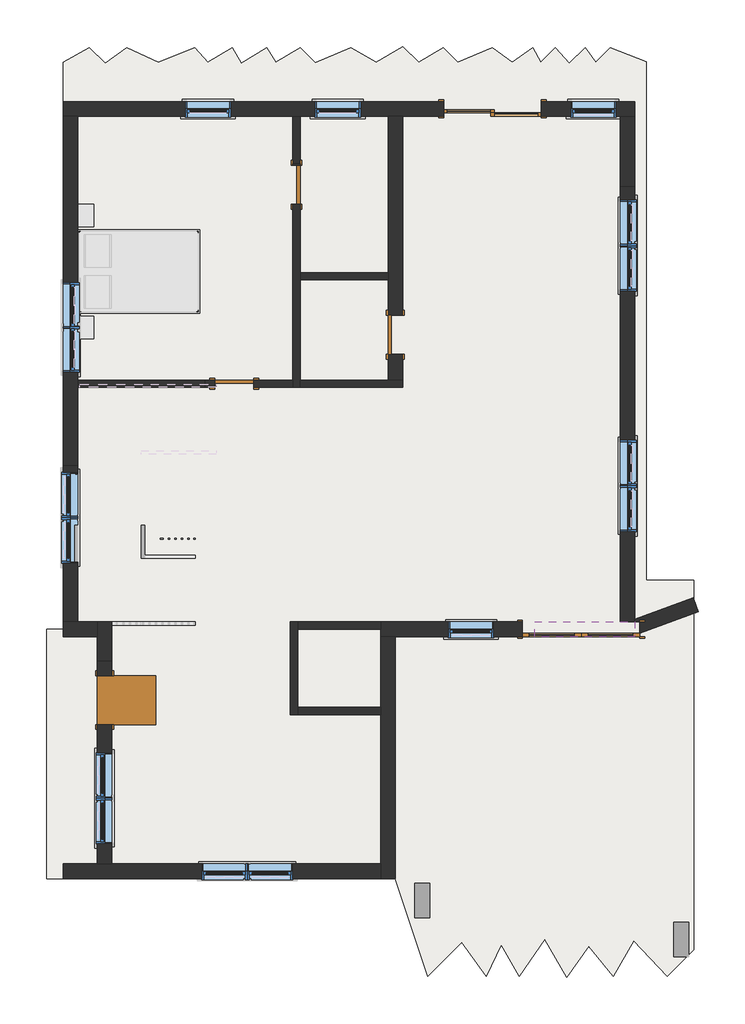
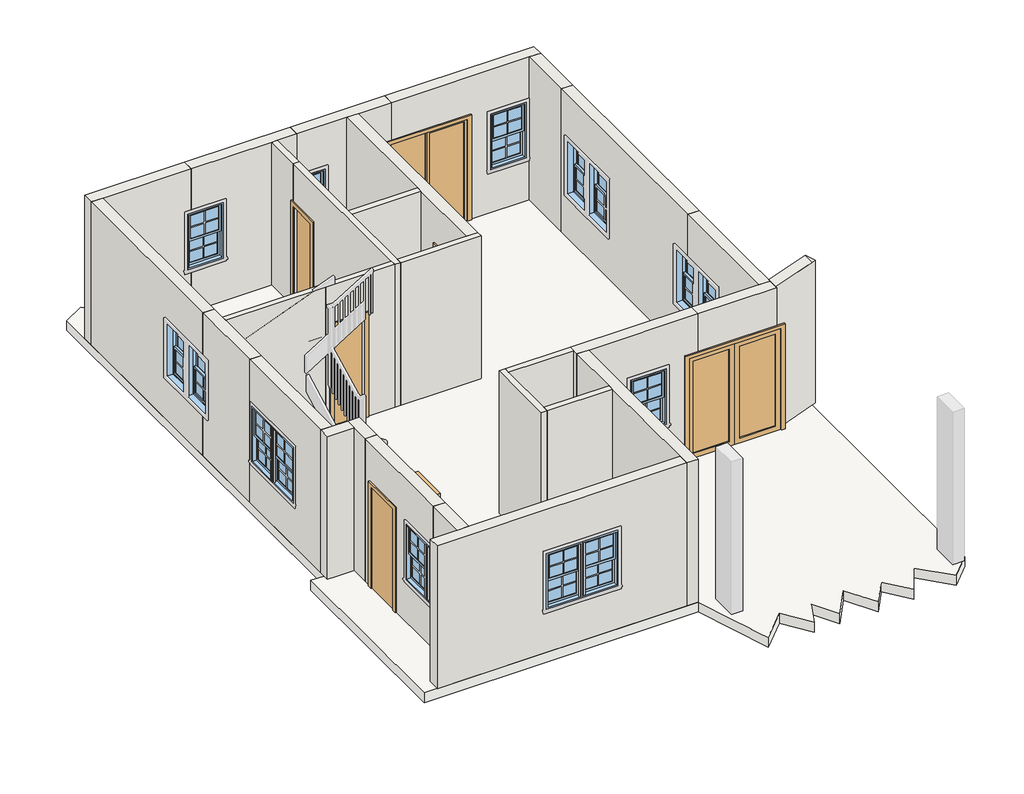
# One storey, part 1 of 3: 29 walls, 16 windows, 6 doors, 1 slab.
"""IFC4 building model written with IfcOpenShell, lengths in millimetres."""

from ifc_helpers import new_model, si_unit, frame, origin, place, context, project, spatial, polyline, outline, extrude, faceted_brep, transform, mapped, element, save
from components import door_5cbd26dd, door_238c678e, single_flush_2_x_7_f433b8c7, door_0bf9f8da, door_0d3b4037, window_fc4bf0c6

model = new_model("IFC4")

# Units and contexts
model_context = context("Model", 3, world=origin())
ifc_project = project(units=[si_unit("LENGTHUNIT", "METRE", prefix="MILLI")], contexts=[model_context])

# Site, building, storey
site = spatial("IfcSite", under=ifc_project)
building = spatial("IfcBuilding", under=site)
storey = spatial("IfcBuildingStorey", under=building, Elevation=3200.4)

# Doors
placement = place(None, origin())
door_shape = door_5cbd26dd(model_context)
element("IfcDoor", 1, ObjectType="Door-Double-Glass : 72\" x 84\"", at=placement, inside=storey, context=model_context, shape_type="MappedRepresentation", body=[
    mapped(door_shape, transform((-14398.9750992, 4551.4036146, 3200.4), x_axis=(-1.0, 0.0, 0.0), y_axis=(0.0, -1.0, 0.0), z_axis=(0.0, 0.0, 1.0))),
])
door_2_shape = door_238c678e(model_context)
element("IfcDoor", 2, ObjectType="Door-Double-Sliding : 60\" x 84\"", at=placement, inside=storey, context=model_context, shape_type="MappedRepresentation", body=[
    mapped(door_2_shape, transform((-15781.8310804, 12791.3223147, 3200.4), x_axis=(-1.0, 0.0, 0.0), y_axis=(0.0, -1.0, 0.0), z_axis=(0.0, 0.0, 1.0))),
])
single_flush_2_x_7_shape = single_flush_2_x_7_f433b8c7(model_context)
element("IfcDoor", 3, ObjectType="Single-Flush : 2' x 7'", at=placement, inside=storey, context=model_context, shape_type="MappedRepresentation", body=[
    mapped(single_flush_2_x_7_shape, transform((-21828.4750314, 3444.1223646, 3200.4), x_axis=(0.0, 1.0, 0.0), y_axis=(-1.0, 0.0, 0.0), z_axis=(0.0, 0.0, 1.0))),
])
door_3_shape = door_0bf9f8da(model_context)
element("IfcDoor", 4, ObjectType="Single-Flush : 24\" x 84\"", at=placement, inside=storey, context=model_context, shape_type="MappedRepresentation", body=[
    mapped(door_3_shape, transform((-18837.6250314, 11478.1423646, 3200.4), x_axis=(0.0, 1.0, 0.0), y_axis=(-1.0, 0.0, 0.0), z_axis=(0.0, 0.0, 1.0))),
])
element("IfcDoor", 5, ObjectType="Single-Flush : 24\" x 84\"", at=placement, inside=storey, context=model_context, shape_type="MappedRepresentation", body=[
    mapped(door_3_shape, transform((-19809.1750314, 8378.0723646, 3200.4), x_axis=(-1.0, 0.0, 0.0), y_axis=(0.0, -1.0, 0.0), z_axis=(0.0, 0.0, 1.0))),
])
door_4_shape = door_0d3b4037(model_context)
element("IfcDoor", 6, ObjectType="Single-Flush : 24\" x 84\"", at=placement, inside=storey, context=model_context, shape_type="MappedRepresentation", body=[
    mapped(door_4_shape, transform((-17294.5750314, 9140.0723646, 3200.4), x_axis=(0.0, 1.0, 0.0), y_axis=(-1.0, 0.0, 0.0), z_axis=(0.0, 0.0, 1.0))),
])

# Slab
element("IfcSlab", 7, ObjectType="LW Concrete on Metal Deck", at=placement, inside=storey, context=model_context, shape_type="SweptSolid", body=[
    extrude(outline(polyline([(-21820.2943548, 13371.8353173), (-21483.0986122, 13616.8223646), (-20992.8643301, 13388.2223646), (-20427.0594754, 13616.8223646), (-20220.0943548, 13388.2223646), (-19839.6400652, 13616.8223646), (-19695.738427, 13377.3298208), (-19297.1559002, 13616.8223646), (-19159.7991627, 13388.2223646), (-18779.344873, 13616.8223646), (-18543.6943548, 13381.1718464), (-17988.5365241, 13616.8223646), (-17592.5897095, 13388.2223646), (-17180.2750314, 13635.9660173), (-16932.5313787, 13388.2223646), (-16552.077089, 13616.8223646), (-16323.477089, 13388.2223646), (-15784.9292382, 13616.8223646), (-15470.2883312, 13388.2223646), (-15155.6474241, 13616.8223646), (-15028.932375, 13388.2223646), (-14800.332375, 13616.8223646), (-14581.2943548, 13373.5559982), (-14338.0279884, 13616.8223646), (-14171.9403665, 13388.2223646), (-13943.3403665, 13616.8223646), (-13382.9750314, 13401.7182659), (-13382.9750314, 5311.0223722), (-12646.3750314, 5311.0223722), (-12646.3750314, -450.2583119), (-13057.2943548, -861.1776354), (-13577.9943548, -311.251504), (-13895.4943548, -861.1776354), (-14276.4943548, -390.1805798), (-14619.3943548, -879.8925313), (-14962.2943548, -285.9723094), (-15365.0574601, -861.1776354), (-15648.0943548, -370.9433534), (-15876.6943548, -861.1776354), (-16257.6943548, -327.7776354), (-16791.0943548, -861.1776354), (-17294.5750314, 662.8223646), (-22734.6943548, 662.8223646), (-22734.6943548, 4549.0223646), (-22476.1752061, 4549.0223646), (-22476.1752061, 13388.2223646), (-22065.2814022, 13616.8223646), (-21820.2943548, 13371.8353173)])), frame((0.0, 0.0, 2997.2), z_axis=(0.0, 0.0, 1.0), x_axis=(1.0, 0.0, 0.0)), (0.0, 0.0, 1.0), 203.2),
])

# Walls
element("IfcWall", 8, ObjectType="Generic - 4.5\"", at=placement, inside=storey, context=model_context, shape_type="SweptSolid", body=[
    extrude(outline(polyline([(-18894.7750314, 11808.3423646), (-18894.7750314, 12550.0223147), (-18780.4750314, 12550.0223147), (-18780.4750314, 11808.3423646), (-18894.7750314, 11808.3423646)])), frame((0.0, 0.0, 3200.4), z_axis=(0.0, 0.0, 1.0), x_axis=(1.0, 0.0, 0.0)), (0.0, 0.0, 1.0), 2997.2),
])
element("IfcWall", 9, ObjectType="Generic - 4.5\"", at=placement, inside=storey, context=model_context, shape_type="Brep", body=[
    faceted_brep([(-18894.7750314, 11808.3423646, 3200.4), (-18894.7750314, 11782.9423646, 3200.4), (-18894.7750314, 11782.9423646, 5334.0), (-18894.7750314, 11173.3423646, 5334.0), (-18894.7750314, 11173.3423646, 3200.4), (-18894.7750314, 8435.2223646, 3200.4), (-18894.7750314, 8320.9223646, 3200.4), (-18894.7750314, 8320.9223646, 6197.6), (-18894.7750314, 8435.2223646, 6197.6), (-18894.7750314, 11808.3423646, 6197.6), (-18780.4750314, 11782.9423646, 5334.0), (-18780.4750314, 11782.9423646, 3200.4), (-18780.4750314, 11808.3423646, 3200.4), (-18780.4750314, 11808.3423646, 6197.6), (-18780.4750314, 10111.6223646, 6197.6), (-18780.4750314, 9997.3223646, 6197.6), (-18780.4750314, 8435.2223646, 6197.6), (-18780.4750314, 8320.9223646, 6197.6), (-18780.4750314, 8320.9223646, 3200.4), (-18780.4750314, 8435.2223646, 3200.4), (-18780.4750314, 9997.3223646, 3200.4), (-18780.4750314, 10111.6223646, 3200.4), (-18780.4750314, 11173.3423646, 3200.4), (-18780.4750314, 11173.3423646, 5334.0)], [[[0, 1, 2, 3, 4, 5, 6, 7, 8, 9]], [[10, 11, 12, 13, 14, 15, 16, 17, 18, 19, 20, 21, 22, 23]], [[12, 11, 1, 0]], [[22, 21, 20, 19, 18, 6, 5, 4]], [[0, 9, 13, 12]], [[7, 6, 18, 17]], [[2, 1, 11, 10]], [[3, 2, 10, 23]], [[4, 3, 23, 22]], [[9, 8, 7, 17, 16, 15, 14, 13]]]),
])
element("IfcWall", 10, ObjectType="Generic - 4.5\"", at=placement, inside=storey, context=model_context, shape_type="Brep", body=[
    faceted_brep([(-18780.4750314, 8320.9223646, 3200.4), (-17180.2750314, 8320.9223646, 3200.4), (-17180.2750314, 8320.9223646, 6197.6), (-18780.4750314, 8320.9223646, 6197.6), (-18780.4750314, 8435.2223646, 3200.4), (-18780.4750314, 8435.2223646, 6197.6), (-17408.8750314, 8435.2223646, 6197.6), (-17180.2750314, 8435.2223646, 6197.6), (-17180.2750314, 8435.2223646, 3200.4), (-17408.8750314, 8435.2223646, 3200.4)], [[[0, 1, 2, 3]], [[4, 5, 6, 7, 8, 9]], [[1, 0, 4, 9, 8]], [[0, 3, 5, 4]], [[2, 1, 8, 7]], [[3, 2, 7, 6, 5]]]),
])
element("IfcWall", 11, ObjectType="Generic - 4.5\"", at=placement, inside=storey, context=model_context, shape_type="SweptSolid", body=[
    extrude(outline(polyline([(3200.4, -20266.3750314), (3200.4, -20113.9750314), (5334.0, -20113.9750314), (5334.0, -19504.3750314), (3200.4, -19504.3750314), (3200.4, -18894.7750314), (6197.6, -18894.7750314), (6197.6, -20266.3750314), (3200.4, -20266.3750314)])), frame((0.0, 8320.9223646, 0.0), z_axis=(0.0, 1.0, 0.0), x_axis=(0.0, 0.0, 1.0)), (0.0, 0.0, 1.0), 114.3),
])
element("IfcWall", 12, ObjectType="Generic - 4.5\"", at=placement, inside=storey, context=model_context, shape_type="SweptSolid", body=[
    extrude(outline(polyline([(-20266.3750314, 8320.9223646), (-22247.5752061, 8320.9223646), (-22247.5752061, 8435.2223646), (-20266.3750314, 8435.2223646), (-20266.3750314, 8320.9223646)])), frame((0.0, 0.0, 3200.4), z_axis=(0.0, 0.0, 1.0), x_axis=(1.0, 0.0, 0.0)), (0.0, 0.0, 1.0), 2997.2),
])
element("IfcWall", 13, ObjectType="Generic - 4.5\"", at=placement, inside=storey, context=model_context, shape_type="SweptSolid", body=[
    extrude(outline(polyline([(-17408.8750314, 9997.3223646), (-18780.4750314, 9997.3223646), (-18780.4750314, 10111.6223646), (-17408.8750314, 10111.6223646), (-17408.8750314, 9997.3223646)])), frame((0.0, 0.0, 3200.4), z_axis=(0.0, 0.0, 1.0), x_axis=(1.0, 0.0, 0.0)), (0.0, 0.0, 1.0), 2997.2),
])
element("IfcWall", 14, ObjectType="Generic - 4.5\"", at=placement, inside=storey, context=model_context, shape_type="Brep", body=[
    faceted_brep([(-18932.8750314, 4663.3223646, 3200.4), (-18932.8750314, 3215.5223646, 3200.4), (-18932.8750314, 3215.5223646, 6197.6), (-18932.8750314, 4663.3223646, 6197.6), (-18818.5750314, 4663.3223646, 3200.4), (-18818.5750314, 4663.3223646, 6197.6), (-18818.5750314, 4549.0223646, 6197.6), (-18818.5750314, 3329.8223646, 6197.6), (-18818.5750314, 3215.5223646, 6197.6), (-18818.5750314, 3215.5223646, 3200.4), (-18818.5750314, 3329.8223646, 3200.4), (-18818.5750314, 4549.0223646, 3200.4)], [[[0, 1, 2, 3]], [[4, 5, 6, 7, 8, 9, 10, 11]], [[1, 0, 4, 11, 10, 9]], [[2, 1, 9, 8]], [[0, 3, 5, 4]], [[3, 2, 8, 7, 6, 5]]]),
])
element("IfcWall", 15, ObjectType="Generic - 4.5\"", at=placement, inside=storey, context=model_context, shape_type="SweptSolid", body=[
    extrude(outline(polyline([(-17523.1750314, 3215.5223646), (-18818.5750314, 3215.5223646), (-18818.5750314, 3329.8223646), (-17523.1750314, 3329.8223646), (-17523.1750314, 3215.5223646)])), frame((0.0, 0.0, 3200.4), z_axis=(0.0, 0.0, 1.0), x_axis=(1.0, 0.0, 0.0)), (0.0, 0.0, 1.0), 2997.2),
])
element("IfcWall", 16, ObjectType="Generic - 4.5\"", at=placement, inside=storey, context=model_context, shape_type="SweptSolid", body=[
    extrude(outline(polyline([(-17523.1750314, 4549.0223646), (-18818.5750314, 4549.0223646), (-18818.5750314, 4663.3223646), (-17523.1750314, 4663.3223646), (-17523.1750314, 4549.0223646)])), frame((0.0, 0.0, 3200.4), z_axis=(0.0, 0.0, 1.0), x_axis=(1.0, 0.0, 0.0)), (0.0, 0.0, 1.0), 2997.2),
])
element("IfcWall", 17, ObjectType="Generic -9\"Brick 2", at=placement, inside=storey, context=model_context, shape_type="Brep", body=[
    faceted_brep([(-22476.1750314, 12550.0223646, 3200.4), (-22247.5750314, 12550.0223646, 3200.4), (-20494.9750314, 12550.0223646, 3200.4), (-20494.9750314, 12550.0223646, 4114.8), (-20571.1750314, 12550.0223646, 4114.8), (-20571.1750314, 12550.0223646, 5283.2), (-20494.9750314, 12550.0223646, 5283.2), (-20494.9750314, 12550.0223646, 6197.6), (-22247.5750314, 12550.0223646, 6197.6), (-22476.1752061, 12550.0223646, 6197.6), (-20494.9750314, 12778.6223646, 3200.4), (-22476.1750314, 12778.6223646, 3200.4), (-22476.1750314, 12778.6223646, 6197.6), (-20494.9750314, 12778.6223646, 6197.6), (-20494.9750314, 12778.6223646, 5283.2), (-20571.1750314, 12778.6223646, 5283.2), (-20571.1750314, 12778.6223646, 4114.8), (-20494.9750314, 12778.6223646, 4114.8)], [[[0, 1, 2, 3, 4, 5, 6, 7, 8, 9]], [[10, 11, 12, 13, 14, 15, 16, 17]], [[2, 1, 0, 11, 10]], [[2, 10, 17, 3]], [[13, 7, 6, 14]], [[0, 9, 12, 11]], [[16, 4, 3, 17]], [[4, 16, 15, 5]], [[5, 15, 14, 6]], [[9, 8, 7, 13, 12]]]),
])
element("IfcWall", 18, ObjectType="Generic -9\"Brick 2", at=placement, inside=storey, context=model_context, shape_type="Brep", body=[
    faceted_brep([(-20494.9750314, 12550.0223147, 3200.4), (-18894.7750314, 12550.0223147, 3200.4), (-18780.4750314, 12550.0223147, 3200.4), (-18397.0494379, 12550.0223147, 3200.4), (-18397.0494379, 12550.0223147, 4114.8), (-18549.4494379, 12550.0223147, 4114.8), (-18549.4494379, 12550.0223147, 5283.2), (-18397.0494379, 12550.0223147, 5283.2), (-18397.0494379, 12550.0223147, 6197.6), (-18780.4750314, 12550.0223147, 6197.6), (-18894.7750314, 12550.0223147, 6197.6), (-20494.9750314, 12550.0223147, 6197.6), (-20494.9750314, 12550.0223147, 5283.2), (-19859.9750314, 12550.0223147, 5283.2), (-19859.9750314, 12550.0223147, 4114.8), (-20494.9750314, 12550.0223147, 4114.8), (-18397.0494379, 12778.6223147, 3200.4), (-20494.9750314, 12778.6223147, 3200.4), (-20494.9750314, 12778.6223147, 4114.8), (-19859.9750314, 12778.6223147, 4114.8), (-19859.9750314, 12778.6223147, 5283.2), (-20494.9750314, 12778.6223147, 5283.2), (-20494.9750314, 12778.6223147, 6197.6), (-18397.0494379, 12778.6223147, 6197.6), (-18397.0494379, 12778.6223147, 5283.2), (-18549.4494379, 12778.6223147, 5283.2), (-18549.4494379, 12778.6223147, 4114.8), (-18397.0494379, 12778.6223147, 4114.8)], [[[0, 1, 2, 3, 4, 5, 6, 7, 8, 9, 10, 11, 12, 13, 14, 15]], [[16, 17, 18, 19, 20, 21, 22, 23, 24, 25, 26, 27]], [[3, 2, 1, 0, 17, 16]], [[3, 16, 27, 4]], [[23, 8, 7, 24]], [[17, 0, 15, 18]], [[12, 11, 22, 21]], [[13, 20, 19, 14]], [[14, 19, 18, 15]], [[20, 13, 12, 21]], [[26, 5, 4, 27]], [[5, 26, 25, 6]], [[6, 25, 24, 7]], [[11, 10, 9, 8, 23, 22]]]),
])
element("IfcWall", 19, ObjectType="Generic -9\"Brick 2", at=placement, inside=storey, context=model_context, shape_type="Brep", body=[
    faceted_brep([(-18397.0494379, 12550.0223147, 4114.8), (-18397.0494379, 12550.0223147, 3200.4), (-17408.8750314, 12550.0223147, 3200.4), (-17180.2750314, 12550.0223147, 3200.4), (-16543.8310804, 12550.0223147, 3200.4), (-16543.8310804, 12550.0223147, 5334.0), (-16518.4310804, 12550.0223147, 5334.0), (-16518.4310804, 12550.0223147, 6197.6), (-17180.2750314, 12550.0223147, 6197.6), (-17408.8750314, 12550.0223147, 6197.6), (-18397.0494379, 12550.0223147, 6197.6), (-18397.0494379, 12550.0223147, 5283.2), (-17838.2494379, 12550.0223147, 5283.2), (-17838.2494379, 12550.0223147, 4114.8), (-18397.0494379, 12778.6223147, 3200.4), (-18397.0494379, 12778.6223147, 4114.8), (-17838.2494379, 12778.6223147, 4114.8), (-17838.2494379, 12778.6223147, 5283.2), (-18397.0494379, 12778.6223147, 5283.2), (-18397.0494379, 12778.6223147, 6197.6), (-16518.4310804, 12778.6223147, 6197.6), (-16518.4310804, 12778.6223147, 5334.0), (-16543.8310804, 12778.6223147, 5334.0), (-16543.8310804, 12778.6223147, 3200.4)], [[[0, 1, 2, 3, 4, 5, 6, 7, 8, 9, 10, 11, 12, 13]], [[14, 15, 16, 17, 18, 19, 20, 21, 22, 23]], [[1, 14, 23, 4, 3, 2]], [[20, 7, 6, 21]], [[14, 1, 0, 15]], [[11, 10, 19, 18]], [[12, 17, 16, 13]], [[13, 16, 15, 0]], [[17, 12, 11, 18]], [[22, 5, 4, 23]], [[5, 22, 21, 6]], [[10, 9, 8, 7, 20, 19]]]),
])
element("IfcWall", 20, ObjectType="Generic -9\"Brick 2", at=placement, inside=storey, context=model_context, shape_type="Brep", body=[
    faceted_brep([(-13560.7750314, 12550.0223147, 3200.4), (-13560.7750314, 12550.0223147, 6197.6), (-13789.3750314, 12550.0223147, 6197.6), (-16518.4310804, 12550.0223147, 6197.6), (-16518.4310804, 12550.0223147, 5334.0), (-15019.8310804, 12550.0223147, 5334.0), (-15019.8310804, 12550.0223147, 3200.4), (-13789.3750314, 12550.0223147, 3200.4), (-13852.8750314, 12550.0223147, 5283.2), (-13852.8750314, 12550.0223147, 4114.8), (-14564.0750314, 12550.0223147, 4114.8), (-14564.0750314, 12550.0223147, 5283.2), (-13560.7750314, 12778.6223147, 6197.6), (-13560.7750314, 12778.6223147, 3200.4), (-15019.8310804, 12778.6223147, 3200.4), (-15019.8310804, 12778.6223147, 5334.0), (-16518.4310804, 12778.6223147, 5334.0), (-16518.4310804, 12778.6223147, 6197.6), (-13852.8750314, 12778.6223147, 5283.2), (-14564.0750314, 12778.6223147, 5283.2), (-14564.0750314, 12778.6223147, 4114.8), (-13852.8750314, 12778.6223147, 4114.8)], [[[0, 1, 2, 3, 4, 5, 6, 7], [8, 9, 10, 11]], [[12, 13, 14, 15, 16, 17], [18, 19, 20, 21]], [[13, 0, 7, 6, 14]], [[3, 17, 16, 4]], [[1, 0, 13, 12]], [[9, 8, 18, 21]], [[10, 9, 21, 20]], [[11, 10, 20, 19]], [[8, 11, 19, 18]], [[5, 15, 14, 6]], [[15, 5, 4, 16]], [[3, 2, 1, 12, 17]]]),
])
element("IfcWall", 21, ObjectType="Generic -9\"Brick 2", at=placement, inside=storey, context=model_context, shape_type="SweptSolid", body=[
    extrude(outline(polyline([(-13789.3750314, 11447.1098201), (-13789.3750314, 12550.0223147), (-13560.7750314, 12550.0223147), (-13560.7750314, 11447.1098201), (-13789.3750314, 11447.1098201)])), frame((0.0, 0.0, 3200.4), z_axis=(0.0, 0.0, 1.0), x_axis=(1.0, 0.0, 0.0)), (0.0, 0.0, 1.0), 2997.2),
])
element("IfcWall", 22, ObjectType="Generic -9\"Brick 2", at=placement, inside=storey, context=model_context, shape_type="SweptSolid", body=[
    extrude(outline(polyline([(11447.1098201, 3200.4), (7101.7223647, 3200.4), (7101.7223647, 4114.8), (7495.4223646, 4114.8), (7495.4223646, 5283.2), (7101.7223647, 5283.2), (7101.7223647, 6197.6), (11447.1098201, 6197.6), (11447.1098201, 3200.4)]), holes=[polyline([(11243.9098201, 4114.8), (11243.9098201, 5283.2), (9821.5098201, 5283.2), (9821.5098201, 4114.8), (11243.9098201, 4114.8)])]), frame((-13789.3750314, 0.0, 0.0), z_axis=(1.0, 0.0, 0.0), x_axis=(0.0, 1.0, 0.0)), (0.0, 0.0, 1.0), 228.6),
])
element("IfcWall", 23, ObjectType="Generic -9\"Brick 2", at=placement, inside=storey, context=model_context, shape_type="Brep", body=[
    faceted_brep([(-13789.3750314, 7101.7223647, 3200.4), (-13789.3750314, 4663.3223646, 3200.4), (-13789.3750314, 4663.3223646, 6197.6), (-13789.3750314, 7101.7223647, 6197.6), (-13789.3750314, 7101.7223647, 5283.2), (-13789.3750314, 6073.0223646, 5283.2), (-13789.3750314, 6073.0223646, 4114.8), (-13789.3750314, 7101.7223647, 4114.8), (-13560.7750314, 4663.3223646, 3200.4), (-13560.7750314, 4704.9241624, 3200.4), (-13560.7750314, 7101.7223647, 3200.4), (-13560.7750314, 7101.7223647, 4114.8), (-13560.7750314, 6073.0223646, 4114.8), (-13560.7750314, 6073.0223646, 5283.2), (-13560.7750314, 7101.7223647, 5283.2), (-13560.7750314, 7101.7223647, 6197.6), (-13560.7750314, 5336.4223722, 6197.6), (-13560.7750314, 4704.9241624, 6197.6), (-13560.7750314, 4663.3223646, 6197.6), (-13560.7750314, 4663.3223646, 5334.0)], [[[0, 1, 2, 3, 4, 5, 6, 7]], [[8, 9, 10, 11, 12, 13, 14, 15, 16, 17, 18, 19]], [[1, 0, 10, 9, 8]], [[10, 0, 7, 11]], [[3, 15, 14, 4]], [[2, 1, 8, 19, 18]], [[6, 12, 11, 7]], [[4, 14, 13, 5]], [[12, 6, 5, 13]], [[15, 3, 2, 18, 17, 16]]]),
])
element("IfcWall", 24, ObjectType="Generic -9\"Brick 2", at=placement, inside=storey, context=model_context, shape_type="Brep", body=[
    faceted_brep([(-13560.7750314, 4434.7223646, 6197.6), (-15122.8751671, 4434.7223646, 6197.6), (-15122.8751671, 4434.7223646, 5334.0), (-13560.7750314, 4434.7223646, 5334.0), (-15122.8751671, 4663.3223646, 6197.6), (-13789.3750314, 4663.3223646, 6197.6), (-13560.7750314, 4663.3223646, 6197.6), (-13560.7750314, 4663.3223646, 5334.0), (-15122.8751671, 4663.3223646, 5334.0), (-13560.7750314, 4461.6531236, 6197.6), (-13560.7750314, 4461.6531236, 5334.0)], [[[0, 1, 2, 3]], [[4, 5, 6, 7, 8]], [[1, 4, 8, 2]], [[6, 9, 0, 3, 10, 7]], [[3, 2, 8, 7, 10]], [[1, 0, 9, 6, 5, 4]]]),
])
element("IfcWall", 25, ObjectType="Generic -9\"Brick 2", at=placement, inside=storey, context=model_context, shape_type="Brep", body=[
    faceted_brep([(-17523.1750314, 4663.3223722, 3200.4), (-17523.1750314, 4663.3223722, 6197.6), (-15122.8751671, 4663.3223722, 6197.6), (-15122.8751671, 4663.3223722, 5334.0), (-15313.3750992, 4663.3223722, 5334.0), (-15313.3750992, 4663.3223722, 3200.4), (-15757.8750314, 4663.3223722, 5283.2), (-16469.0750314, 4663.3223722, 5283.2), (-16469.0750314, 4663.3223722, 4114.8), (-15757.8750314, 4663.3223722, 4114.8), (-17523.1750314, 4434.7223722, 6197.6), (-17523.1750314, 4434.7223722, 3200.4), (-17294.5750314, 4434.7223722, 3200.4), (-15313.3750992, 4434.7223722, 3200.4), (-15313.3750992, 4434.7223722, 5334.0), (-15122.8751671, 4434.7223722, 5334.0), (-15122.8751671, 4434.7223722, 6197.6), (-17294.5750314, 4434.7223722, 6197.6), (-15757.8750314, 4434.7223722, 5283.2), (-15757.8750314, 4434.7223722, 4114.8), (-16469.0750314, 4434.7223722, 4114.8), (-16469.0750314, 4434.7223722, 5283.2), (-17523.1750314, 4549.0223646, 3200.4), (-17523.1750314, 4549.0223646, 6197.6)], [[[0, 1, 2, 3, 4, 5], [6, 7, 8, 9]], [[10, 11, 12, 13, 14, 15, 16, 17], [18, 19, 20, 21]], [[11, 22, 0, 5, 13, 12]], [[2, 16, 15, 3]], [[1, 0, 22, 11, 10, 23]], [[4, 14, 13, 5]], [[14, 4, 3, 15]], [[19, 18, 6, 9]], [[20, 19, 9, 8]], [[21, 20, 8, 7]], [[18, 21, 7, 6]], [[2, 1, 23, 10, 17, 16]]]),
])
element("IfcWall", 26, ObjectType="Generic -9\"Brick 2", at=placement, inside=storey, context=model_context, shape_type="Brep", body=[
    faceted_brep([(-17523.1750314, 4434.7223722, 3200.4), (-17523.1750314, 3329.8223646, 3200.4), (-17523.1750314, 3215.5223646, 3200.4), (-17523.1750314, 891.4223646, 3200.4), (-17523.1750314, 662.8223646, 3200.4), (-17523.1750314, 662.8223646, 6197.6), (-17523.1750314, 891.4223646, 6197.6), (-17523.1750314, 3215.5223646, 6197.6), (-17523.1750314, 3329.8223646, 6197.6), (-17523.1750314, 4434.7223722, 6197.6), (-17294.5750314, 4434.7223722, 3200.4), (-17294.5750314, 4434.7223722, 6197.6), (-17294.5750314, 662.8223646, 6197.6), (-17294.5750314, 662.8223646, 3200.4)], [[[0, 1, 2, 3, 4, 5, 6, 7, 8, 9]], [[10, 11, 12, 13]], [[4, 3, 2, 1, 0, 10, 13]], [[0, 9, 11, 10]], [[5, 4, 13, 12]], [[9, 8, 7, 6, 5, 12, 11]]]),
])
element("IfcWall", 27, ObjectType="Generic -9\"Brick 2", at=placement, inside=storey, context=model_context, shape_type="Brep", body=[
    faceted_brep([(-17523.1750314, 891.4223646, 3200.4), (-21714.1750314, 891.4223646, 3200.4), (-21942.7750314, 891.4223646, 3200.4), (-22476.1750314, 891.4223646, 3200.4), (-22476.1750314, 891.4223646, 6197.6), (-21942.7750314, 891.4223646, 6197.6), (-21714.1750314, 891.4223646, 6197.6), (-17523.1750314, 891.4223646, 6197.6), (-18894.6931686, 891.4223646, 5283.2), (-20317.0931686, 891.4223646, 5283.2), (-20317.0931686, 891.4223646, 4114.8), (-18894.6931686, 891.4223646, 4114.8), (-22476.1750314, 662.8223646, 3200.4), (-17523.1750314, 662.8223646, 3200.4), (-17523.1750314, 662.8223646, 6197.6), (-22476.1750314, 662.8223646, 6197.6), (-20317.0931686, 662.8223646, 5283.2), (-18894.6931686, 662.8223646, 5283.2), (-18894.6931686, 662.8223646, 4114.8), (-20317.0931686, 662.8223646, 4114.8)], [[[0, 1, 2, 3, 4, 5, 6, 7], [8, 9, 10, 11]], [[12, 13, 14, 15], [16, 17, 18, 19]], [[3, 2, 1, 0, 13, 12]], [[4, 3, 12, 15]], [[0, 7, 14, 13]], [[16, 9, 8, 17]], [[18, 11, 10, 19]], [[18, 17, 8, 11]], [[19, 10, 9, 16]], [[7, 6, 5, 4, 15, 14]]]),
])
element("IfcWall", 28, ObjectType="Generic -9\"Brick 2", at=placement, inside=storey, context=model_context, shape_type="SweptSolid", body=[
    extrude(outline(polyline([(1710.5723646, 3200.4), (891.4223646, 3200.4), (891.4223646, 6197.6), (1710.5723646, 6197.6), (1710.5723646, 5283.2), (1202.5723646, 5283.2), (1202.5723646, 4114.8), (1710.5723646, 4114.8), (1710.5723646, 3200.4)])), frame((-21942.7750314, 0.0, 0.0), z_axis=(1.0, 0.0, 0.0), x_axis=(0.0, 1.0, 0.0)), (0.0, 0.0, 1.0), 228.6),
])
element("IfcWall", 29, ObjectType="Generic -9\"Brick 2", at=placement, inside=storey, context=model_context, shape_type="SweptSolid", body=[
    extrude(outline(polyline([(4053.7223646, 3200.4), (3825.1223646, 3200.4), (3825.1223646, 5334.0), (3063.1223646, 5334.0), (3063.1223646, 3200.4), (1710.5723646, 3200.4), (1710.5723646, 4114.8), (2624.9723646, 4114.8), (2624.9723646, 5283.2), (1710.5723646, 5283.2), (1710.5723646, 6197.6), (4053.7223646, 6197.6), (4053.7223646, 3200.4)])), frame((-21942.7750314, 0.0, 0.0), z_axis=(1.0, 0.0, 0.0), x_axis=(0.0, 1.0, 0.0)), (0.0, 0.0, 1.0), 228.6),
])
element("IfcWall", 30, ObjectType="Generic -9\"Brick 2", at=placement, inside=storey, context=model_context, shape_type="Brep", body=[
    faceted_brep([(-21714.1750314, 4053.7223646, 3200.4), (-21714.1750314, 4663.3223646, 3200.4), (-21714.1750314, 4663.3223646, 6197.6), (-21714.1750314, 4053.7223646, 6197.6), (-21942.7750314, 4053.7223646, 3200.4), (-21942.7750314, 4053.7223646, 6197.6), (-21942.7750314, 4434.7223646, 6197.6), (-21942.7750314, 4663.3223646, 6197.6), (-21942.7750314, 4663.3223646, 3200.4), (-21942.7750314, 4434.7223646, 3200.4)], [[[0, 1, 2, 3]], [[4, 5, 6, 7, 8, 9]], [[1, 0, 4, 9, 8]], [[0, 3, 5, 4]], [[2, 1, 8, 7]], [[3, 2, 7, 6, 5]]]),
])
element("IfcWall", 31, ObjectType="Generic -9\"Brick 2", at=placement, inside=storey, context=model_context, shape_type="SweptSolid", body=[
    extrude(outline(polyline([(12550.0223646, 3200.4), (8710.539033, 3200.4), (8710.539033, 4114.8), (9955.139033, 4114.8), (9955.139033, 5283.2), (8710.539033, 5283.2), (8710.539033, 6197.6), (12550.0223646, 6197.6), (12550.0223646, 3200.4)])), frame((-22476.1750314, 0.0, 0.0), z_axis=(1.0, 0.0, 0.0), x_axis=(0.0, 1.0, 0.0)), (0.0, 0.0, 1.0), 228.6),
])
element("IfcWall", 32, ObjectType="Generic -9\"Brick 2", at=placement, inside=storey, context=model_context, shape_type="Brep", body=[
    faceted_brep([(-22476.1752061, 8710.539033, 3200.4), (-22476.1752061, 7101.7223643, 3200.4), (-22476.1752061, 7101.7223643, 6197.6), (-22476.1752061, 8710.539033, 6197.6), (-22476.1752061, 8710.539033, 5283.2), (-22476.1752061, 8558.139033, 5283.2), (-22476.1752061, 8558.139033, 4114.8), (-22476.1752061, 8710.539033, 4114.8), (-22247.5752061, 7101.7223643, 3200.4), (-22247.5752061, 8320.9223646, 3200.4), (-22247.5752061, 8435.2223646, 3200.4), (-22247.5752061, 8710.539033, 3200.4), (-22247.5752061, 8710.539033, 4114.8), (-22247.5752061, 8558.139033, 4114.8), (-22247.5752061, 8558.139033, 5283.2), (-22247.5752061, 8710.539033, 5283.2), (-22247.5752061, 8710.539033, 6197.6), (-22247.5752061, 8435.2223646, 6197.6), (-22247.5752061, 8320.9223646, 6197.6), (-22247.5752061, 7101.7223643, 6197.6)], [[[0, 1, 2, 3, 4, 5, 6, 7]], [[8, 9, 10, 11, 12, 13, 14, 15, 16, 17, 18, 19]], [[1, 0, 11, 10, 9, 8]], [[2, 1, 8, 19]], [[11, 0, 7, 12]], [[3, 16, 15, 4]], [[6, 13, 12, 7]], [[13, 6, 5, 14]], [[14, 5, 4, 15]], [[3, 2, 19, 18, 17, 16]]]),
])
element("IfcWall", 33, ObjectType="Generic -9\"Brick 2", at=placement, inside=storey, context=model_context, shape_type="SweptSolid", body=[
    extrude(outline(polyline([(7101.7223643, 3200.4), (4663.3223646, 3200.4), (4663.3223646, 6197.6), (7101.7223643, 6197.6), (7101.7223643, 3200.4)]), holes=[polyline([(5577.7223643, 4114.8), (7000.1223643, 4114.8), (7000.1223643, 5283.2), (5577.7223643, 5283.2), (5577.7223643, 4114.8)])]), frame((-22476.1752061, 0.0, 0.0), z_axis=(1.0, 0.0, 0.0), x_axis=(0.0, 1.0, 0.0)), (0.0, 0.0, 1.0), 228.6),
])
element("IfcWall", 34, ObjectType="Generic -9\"Brick 2", at=placement, inside=storey, context=model_context, shape_type="Brep", body=[
    faceted_brep([(-22476.1752061, 4434.7223646, 3200.4), (-21942.7750314, 4434.7223646, 3200.4), (-21942.7750314, 4434.7223646, 6197.6), (-22476.1752061, 4434.7223646, 6197.6), (-22476.1752061, 4663.3223646, 3200.4), (-22476.1752061, 4663.3223646, 6197.6), (-22247.5752061, 4663.3223646, 6197.6), (-21942.7750314, 4663.3223646, 6197.6), (-21942.7750314, 4663.3223646, 3200.4), (-22247.5752061, 4663.3223646, 3200.4)], [[[0, 1, 2, 3]], [[4, 5, 6, 7, 8, 9]], [[1, 0, 4, 9, 8]], [[0, 3, 5, 4]], [[2, 1, 8, 7]], [[3, 2, 7, 6, 5]]]),
])
element("IfcWall", 35, ObjectType="Generic -9\"Brick 2", at=placement, inside=storey, context=model_context, shape_type="Brep", body=[
    faceted_brep([(-17408.8750314, 12550.0223147, 3200.4), (-17408.8750314, 10111.6223646, 3200.4), (-17408.8750314, 9997.3223646, 3200.4), (-17408.8750314, 9444.8723646, 3200.4), (-17408.8750314, 9444.8723646, 5334.0), (-17408.8750314, 8835.2723646, 5334.0), (-17408.8750314, 8835.2723646, 3200.4), (-17408.8750314, 8435.2223646, 3200.4), (-17408.8750314, 8435.2223646, 6197.6), (-17408.8750314, 9997.3223646, 6197.6), (-17408.8750314, 10111.6223646, 6197.6), (-17408.8750314, 12550.0223147, 6197.6), (-17180.2750314, 9444.8723646, 5334.0), (-17180.2750314, 9444.8723646, 3200.4), (-17180.2750314, 12550.0223147, 3200.4), (-17180.2750314, 12550.0223147, 6197.6), (-17180.2750314, 8435.2223646, 6197.6), (-17180.2750314, 8435.2223646, 3200.4), (-17180.2750314, 8835.2723646, 3200.4), (-17180.2750314, 8835.2723646, 5334.0)], [[[0, 1, 2, 3, 4, 5, 6, 7, 8, 9, 10, 11]], [[12, 13, 14, 15, 16, 17, 18, 19]], [[18, 17, 7, 6]], [[14, 13, 3, 2, 1, 0]], [[0, 11, 15, 14]], [[8, 7, 17, 16]], [[4, 3, 13, 12]], [[5, 4, 12, 19]], [[6, 5, 19, 18]], [[11, 10, 9, 8, 16, 15]]]),
])
element("IfcWall", 36, ObjectType="Generic -9\"Brick 2", at=placement, inside=storey, context=model_context, shape_type="Brep", body=[
    faceted_brep([(-12570.5569462, 4822.063032, 3200.4), (-12570.5569462, 4822.063032, 6197.6), (-12646.3750314, 4794.4675058, 6197.6), (-13560.7750314, 4461.6531236, 6197.6), (-13560.7750314, 4461.6531236, 5334.0), (-13484.5750992, 4489.3876307, 5334.0), (-13484.5750992, 4489.3876307, 3200.4), (-12648.7427509, 5036.8767651, 3200.4), (-13560.7750314, 4704.9241624, 3200.4), (-13560.7750314, 4704.9241624, 6197.6), (-12648.7427509, 5036.8767651, 6197.6), (-13484.5750992, 4663.3223646, 3200.4), (-13560.7750314, 4663.3223646, 3200.4), (-12646.3750314, 5030.3715091, 6197.6), (-13560.7750314, 4663.3223646, 5334.0), (-13560.7750314, 4663.3223646, 6197.6), (-13484.5750992, 4663.3223646, 5334.0)], [[[0, 1, 2, 3, 4, 5, 6]], [[7, 8, 9, 10]], [[8, 7, 0, 6, 11, 12]], [[1, 0, 7, 10, 13]], [[9, 8, 12, 14, 4, 3, 15]], [[16, 5, 4, 14]], [[16, 11, 6, 5]], [[11, 16, 14, 12]], [[2, 1, 13]], [[3, 2, 13, 10, 9, 15]]]),
])

# Windows
window_shape = window_fc4bf0c6(model_context)
element("IfcWindow", 37, ObjectType="Window-Double-Hung : 28\" x 46\"", at=placement, inside=storey, context=model_context, shape_type="MappedRepresentation", body=[
    mapped(window_shape, transform((-20215.5750314, 12664.3223147, 3200.4), x_axis=(-1.0, 0.0, 0.0), y_axis=(0.0, -1.0, 0.0), z_axis=(0.0, 0.0, 1.0))),
])
element("IfcWindow", 38, ObjectType="Window-Double-Hung : 28\" x 46\"", at=placement, inside=storey, context=model_context, shape_type="MappedRepresentation", body=[
    mapped(window_shape, transform((-14208.4750314, 12664.3223147, 3200.4), x_axis=(-1.0, 0.0, 0.0), y_axis=(0.0, -1.0, 0.0), z_axis=(0.0, 0.0, 1.0))),
])
element("IfcWindow", 39, ObjectType="Window-Double-Hung : 28\" x 46\"", at=placement, inside=storey, context=model_context, shape_type="MappedRepresentation", body=[
    mapped(window_shape, transform((-13675.0750314, 10888.3098201, 3200.4), x_axis=(0.0, -1.0, 0.0), y_axis=(1.0, 0.0, 0.0), z_axis=(0.0, 0.0, 1.0))),
])
element("IfcWindow", 40, ObjectType="Window-Double-Hung : 28\" x 46\"", at=placement, inside=storey, context=model_context, shape_type="MappedRepresentation", body=[
    mapped(window_shape, transform((-13675.0750314, 10177.1098201, 3200.4), x_axis=(0.0, -1.0, 0.0), y_axis=(1.0, 0.0, 0.0), z_axis=(0.0, 0.0, 1.0))),
])
element("IfcWindow", 41, ObjectType="Window-Double-Hung : 28\" x 46\"", at=placement, inside=storey, context=model_context, shape_type="MappedRepresentation", body=[
    mapped(window_shape, transform((-13675.0750314, 7139.8223646, 3200.4), x_axis=(0.0, -1.0, 0.0), y_axis=(1.0, 0.0, 0.0), z_axis=(0.0, 0.0, 1.0))),
])
element("IfcWindow", 42, ObjectType="Window-Double-Hung : 28\" x 46\"", at=placement, inside=storey, context=model_context, shape_type="MappedRepresentation", body=[
    mapped(window_shape, transform((-13675.0750314, 6428.6223646, 3200.4), x_axis=(0.0, -1.0, 0.0), y_axis=(1.0, 0.0, 0.0), z_axis=(0.0, 0.0, 1.0))),
])
element("IfcWindow", 43, ObjectType="Window-Double-Hung : 28\" x 46\"", at=placement, inside=storey, context=model_context, shape_type="MappedRepresentation", body=[
    mapped(window_shape, transform((-19961.4931686, 777.1223646, 3200.4), x_axis=(-1.0, 0.0, 0.0), y_axis=(0.0, -1.0, 0.0), z_axis=(0.0, 0.0, 1.0))),
])
element("IfcWindow", 44, ObjectType="Window-Double-Hung : 28\" x 46\"", at=placement, inside=storey, context=model_context, shape_type="MappedRepresentation", body=[
    mapped(window_shape, transform((-19250.2931686, 777.1223646, 3200.4), x_axis=(-1.0, 0.0, 0.0), y_axis=(0.0, -1.0, 0.0), z_axis=(0.0, 0.0, 1.0))),
])
element("IfcWindow", 45, ObjectType="Window-Double-Hung : 28\" x 46\"", at=placement, inside=storey, context=model_context, shape_type="MappedRepresentation", body=[
    mapped(window_shape, transform((-21828.4750314, 2269.3723646, 3200.4), x_axis=(0.0, 1.0, 0.0), y_axis=(-1.0, 0.0, 0.0), z_axis=(0.0, 0.0, 1.0))),
])
element("IfcWindow", 46, ObjectType="Window-Double-Hung : 28\" x 46\"", at=placement, inside=storey, context=model_context, shape_type="MappedRepresentation", body=[
    mapped(window_shape, transform((-21828.4750314, 1558.1723646, 3200.4), x_axis=(0.0, 1.0, 0.0), y_axis=(-1.0, 0.0, 0.0), z_axis=(0.0, 0.0, 1.0))),
])
element("IfcWindow", 47, ObjectType="Window-Double-Hung : 28\" x 46\"", at=placement, inside=storey, context=model_context, shape_type="MappedRepresentation", body=[
    mapped(window_shape, transform((-22361.8752061, 6644.5223643, 3200.4), x_axis=(0.0, 1.0, 0.0), y_axis=(-1.0, 0.0, 0.0), z_axis=(0.0, 0.0, 1.0))),
])
element("IfcWindow", 48, ObjectType="Window-Double-Hung : 28\" x 46\"", at=placement, inside=storey, context=model_context, shape_type="MappedRepresentation", body=[
    mapped(window_shape, transform((-22361.8752061, 5933.3223643, 3200.4), x_axis=(0.0, 1.0, 0.0), y_axis=(-1.0, 0.0, 0.0), z_axis=(0.0, 0.0, 1.0))),
])
element("IfcWindow", 49, ObjectType="Window-Double-Hung : 28\" x 46\"", at=placement, inside=storey, context=model_context, shape_type="MappedRepresentation", body=[
    mapped(window_shape, transform((-22361.8750314, 9599.539033, 3200.4), x_axis=(0.0, -1.0, 0.0), y_axis=(1.0, 0.0, 0.0), z_axis=(0.0, 0.0, 1.0))),
])
element("IfcWindow", 50, ObjectType="Window-Double-Hung : 28\" x 46\"", at=placement, inside=storey, context=model_context, shape_type="MappedRepresentation", body=[
    mapped(window_shape, transform((-22361.8750314, 8913.739033, 3200.4), x_axis=(0.0, -1.0, 0.0), y_axis=(1.0, 0.0, 0.0), z_axis=(0.0, 0.0, 1.0))),
])
element("IfcWindow", 51, ObjectType="Window-Double-Hung : 28\" x 46\"", at=placement, inside=storey, context=model_context, shape_type="MappedRepresentation", body=[
    mapped(window_shape, transform((-18193.8494379, 12664.3223147, 3200.4), x_axis=(-1.0, 0.0, 0.0), y_axis=(0.0, -1.0, 0.0), z_axis=(0.0, 0.0, 1.0))),
])
element("IfcWindow", 52, ObjectType="Window-Double-Hung : 28\" x 46\"", at=placement, inside=storey, context=model_context, shape_type="MappedRepresentation", body=[
    mapped(window_shape, transform((-16113.4750314, 4549.0223722, 3200.4), x_axis=(-1.0, 0.0, 0.0), y_axis=(0.0, -1.0, 0.0), z_axis=(0.0, 0.0, 1.0))),
])

save(model, "model.ifc")

# Revit data of these elements
# Type "Door-Double-Glass : 72\" x 84\""
#   Type Mark = "13"
#   Construction Type Id = "opn-d45"
#   Assembly Code = "C1020"
#   Analytic Construction = "Wood frame, double glass door "
#   W = 3' - 0"
#   Thickness = 0' - 2"
#   Thermal Resistance (R) = 1.8150 (h·ft²·°F)/BTU
#   Swing Angle [instance default] = 90.00°
#   Heat Transfer Coefficient (U) = 0.5510 BTU/(h·ft²·°F)
#   Height = 7' - 0"
#   Bottom Rail = 0' - 4"
#   Top Rail = 0' - 4"
#   Stiles = 0' - 4"
#   Trim Projection = 0' - 1"
#   Trim Width = 0' - 3"
#   Width = 6' - 0"
#   Define Thermal Properties by = 1
#   Glazing = Glass
#   Panel Material = Wood - Birch - Solid Stained Light Low Gloss
#   Trim Material = Paint - Sienna
#   Visual Light Transmittance = 0
#   Solar Heat Gain Coefficient = 0
#   Function = (empty or 0)
#   Wall Closure = (empty or 0)
# Type "Door-Double-Sliding : 60\" x 84\""
#   Type Mark = "9"
#   Construction Type Id = "opn-d45"
#   Assembly Code = "C1020"
#   Analytic Construction = "Wood frame, double glass door "
#   Thickness = 0' - 2"
#   Thermal Resistance (R) = 1.8150 (h·ft²·°F)/BTU
#   Heat Transfer Coefficient (U) = 0.5510 BTU/(h·ft²·°F)
#   Height = 7' - 0"
#   Rail Width = 0' - 2"
#   Stiles = 0' - 2"
#   Trim Projection Ext = 0' - 1"
#   Trim Projection Int = 0' - 1"
#   Trim Width = 0' - 3"
#   Width = 5' - 0"
#   Define Thermal Properties by = 1
#   Glazing = Glass
#   Panel Material = Wood - Birch - Solid Stained Light Low Gloss
#   Trim Material = Paint - Sienna
#   Visual Light Transmittance = 0
#   Solar Heat Gain Coefficient = 0
#   Function = (empty or 0)
#   Wall Closure = (empty or 0)
# Type "Single-Flush : 2' x 7'"
#   Type Mark = "10"
#   Construction Type Id = "MDOOR"
#   Assembly Code = "C1020"
#   Analytic Construction = "Metal"
#   Thickness = 3' - 0"
#   Heat Transfer Coefficient (U) = 0.651978 BTU/(h·ft²·°F)
#   Height = 7' - 0"
#   Trim Projection Ext = 0' - 1"
#   Trim Projection Int = 0' - 1"
#   Trim Width = 0' - 3"
#   Width = 2' - 6"
#   Define Thermal Properties by = 1
#   Door Material = Door - Panel
#   Frame Material = Door - Frame
#   Visual Light Transmittance = 0
#   Solar Heat Gain Coefficient = 0
#   Function = (empty or 0)
#   Wall Closure = (empty or 0)
# Type "Single-Flush : 24\" x 84\""
#   Type Mark = "1"
#   Construction Type Id = "MDOOR"
#   Assembly Code = "C1020"
#   Analytic Construction = "Metal"
#   Thickness = 0' - 2"
#   Heat Transfer Coefficient (U) = 0.651978 BTU/(h·ft²·°F)
#   Height = 7' - 0"
#   Trim Projection Ext = 0' - 1"
#   Trim Projection Int = 0' - 1"
#   Trim Width = 0' - 3"
#   Width = 2' - 0"
#   Define Thermal Properties by = 1
#   Define Thermal Properties by = 1
#   Door Material = Door - Panel
#   Frame Material = Door - Frame
#   Visual Light Transmittance = 0
#   Solar Heat Gain Coefficient = 0
#   Function = (empty or 0)
#   Wall Closure = (empty or 0)
# Type "LW Concrete on Metal Deck"
#   Assembly Code = "B1010"
#   Function = 0
#   Layers, outside or top first: 0' - 6" "Concrete, Lightweight" (function 1); 0' - 2" "Metal Deck" (function 1)
# Type "Generic - 4.5\""
#   Assembly Code = "B2010"
#   Layers, outside or top first: 0' - 4 1/2" no material (function 1)
# Type "Generic -9\"Brick 2"
#   Assembly Code = "B2010"
#   Layers, outside or top first: 0' - 9" "Brick, Common" (function 1)
# Type "Window-Double-Hung : 28\" x 46\""
#   Type Mark = "12"
#   Fire Rating = "0.5h"
#   Construction Type Id = "DG-DR"
#   Assembly Code = "B2020100"
#   Analytic Construction = "Double glazing - domestic"
#   Wall Thickness [instance default] = 0' - 6"
#   Window Inset [instance default] = 0' - 0"
#   Visual Light Transmittance = 0.81
#   Thermal Resistance (R) = 1.8146 (h·ft²·°F)/BTU
#   Solar Heat Gain Coefficient = 0.76
#   Muntin Width = 1' - 10"
#   Muntin Height = 1' - 7 1/8"
#   Interior Wall Closure [instance default] = 0' - 1 1/2"
#   Rough Width = 2' - 4 1/2"
#   Rough Height = 3' - 10 1/2"
#   Frame Extension [instance default] = 0' - 1 1/4"
#   Exterior Wall Closure [instance default] = 0' - 0 1/2"
#   Extension Jamb [instance default] = 0' - 1 1/2"
#   Heat Transfer Coefficient (U) = 0.5511 BTU/(h·ft²·°F)
#   Height = 3' - 10"
#   Width = 2' - 4"
#   Define Thermal Properties by = 1
#   Top Muntin Visibility = yes
#   Indicator Visibility [instance default] = yes
#   Extension Jamb Visibility [instance default] = yes
#   Interior Trim Visibility [instance default] = yes
#   Exterior Trim Visibility [instance default] = yes
#   Define Thermal Properties by = 1
#   Bottom Muntin Visibility = yes
#   Muntin Pattern = Muntin Pattern_2x2 : Muntin Pattern_2x2
#   Interior Trim Material = Wood - Stained
#   Interior Trim = Trim-Window-Interior-Flat : Picture Frame
#   Exterior Trim Material = Clad - White
#   Exterior Trim = Trim-Window-Exterior-Flat : with Sill
#   Glass Panel Material = Glass
#   Exterior Frame Material = Clad - White
#   Interior Frame Material = Wood - Stained
#   Wall Closure = (empty or 0)
# Element 1 (IfcDoor, "Door-Double-Glass : 72\" x 84\"")
#   Swing Angle = 90.00°
#   Phase Created = New Construction
#   Materials on its faces: "Wood - Birch - Solid Stained Light Low Gloss", "Paint - Sienna", "Glass"
# Element 2 (IfcDoor, "Door-Double-Sliding : 60\" x 84\"")
#   Phase Created = New Construction
#   Materials on its faces: "Paint - Sienna", "Wood - Birch - Solid Stained Light Low Gloss", "Glass"
# Element 3 (IfcDoor, "Single-Flush : 2' x 7'")
#   Phase Created = New Construction
#   Materials on its faces: "Door - Frame", "Door - Panel"
# Elements 4, 5, 6 (IfcDoor, "Single-Flush : 24\" x 84\"")
#   Phase Created = New Construction
#   Materials on its faces: "Door - Frame", "Door - Panel"
# Element 7 (IfcSlab, "LW Concrete on Metal Deck")
#   built-in parameter 1001955 = 0.507704 (stored number, unit not read)
#   Height Offset From Level = 0' - 0"
#   Phase Created = New Construction
#   Materials on its faces: "Metal Deck", "Concrete, Lightweight"
# Elements 8, 9, 11, 12, 13, 14, 15, 16 (IfcWall, "Generic - 4.5\"")
#   Top Offset = -0' - 6"
#   Base Offset = 0' - 0"
#   wall height = 9' - 10"
#   Phase Created = New Construction
#   Top Constraint = 2 ND FLOOR
#   Materials on its faces: "Default Wall"
# Element 10 (IfcWall, "Generic - 4.5\"")
#   Top Offset = -0' - 6"
#   Base Offset = 0' - 0"
#   wall height = 9' - 10"
#   Phase Created = New Construction
#   Top Constraint = 2 ND FLOOR
#   Materials on its faces: "Default Wall", "Brick, Common"
# Elements 17, 18, 19, 20, 21, 22, 24, 25, 26, 27, 28, 29, 30, 31, 32, 33, 34, 35, 36 (IfcWall, "Generic -9\"Brick 2")
#   Top Offset = -0' - 6"
#   Base Offset = 0' - 0"
#   wall height = 9' - 10"
#   Phase Created = New Construction
#   Top Constraint = 2 ND FLOOR
#   Materials on its faces: "Brick, Common"
# Element 23 (IfcWall, "Generic -9\"Brick 2")
#   Top Offset = 0' - 0"
#   Base Offset = 0' - 0"
#   wall height = 9' - 10"
#   Phase Created = New Construction
#   Top Constraint = 2 ND FLOOR
#   Materials on its faces: "Brick, Common"
# Element 37 (IfcWindow, "Window-Double-Hung : 28\" x 46\"")
#   Mark = "17"
#   Window Inset = 0' - 0"
#   Interior Wall Closure = 0' - 1 1/2"
#   Frame Extension = 0' - 1 1/4"
#   Exterior Wall Closure = 0' - 0 1/2"
#   Interior Trim Visibility = yes
#   Indicator Visibility = yes
#   Exterior Trim Visibility = yes
#   Phase Created = New Construction
#   Materials on its faces: "Wood - Stained", "Glass", "Clad - White"
# Element 38 (IfcWindow, "Window-Double-Hung : 28\" x 46\"")
#   Mark = "18"
#   Window Inset = 0' - 0"
#   Interior Wall Closure = 0' - 1 1/2"
#   Frame Extension = 0' - 1 1/4"
#   Exterior Wall Closure = 0' - 0 1/2"
#   Interior Trim Visibility = yes
#   Indicator Visibility = yes
#   Exterior Trim Visibility = yes
#   Phase Created = New Construction
#   Materials on its faces: "Wood - Stained", "Glass", "Clad - White"
# Element 39 (IfcWindow, "Window-Double-Hung : 28\" x 46\"")
#   Mark = "19"
#   Window Inset = 0' - 0"
#   Interior Wall Closure = 0' - 1 1/2"
#   Frame Extension = 0' - 1 1/4"
#   Exterior Wall Closure = 0' - 0 1/2"
#   Interior Trim Visibility = yes
#   Indicator Visibility = yes
#   Exterior Trim Visibility = yes
#   Phase Created = New Construction
#   Materials on its faces: "Wood - Stained", "Glass", "Clad - White"
# Element 40 (IfcWindow, "Window-Double-Hung : 28\" x 46\"")
#   Mark = "20"
#   Window Inset = 0' - 0"
#   Interior Wall Closure = 0' - 1 1/2"
#   Frame Extension = 0' - 1 1/4"
#   Exterior Wall Closure = 0' - 0 1/2"
#   Interior Trim Visibility = yes
#   Indicator Visibility = yes
#   Exterior Trim Visibility = yes
#   Phase Created = New Construction
#   Materials on its faces: "Wood - Stained", "Glass", "Clad - White"
# Element 41 (IfcWindow, "Window-Double-Hung : 28\" x 46\"")
#   Mark = "21"
#   Window Inset = 0' - 0"
#   Interior Wall Closure = 0' - 1 1/2"
#   Frame Extension = 0' - 1 1/4"
#   Exterior Wall Closure = 0' - 0 1/2"
#   Interior Trim Visibility = yes
#   Indicator Visibility = yes
#   Exterior Trim Visibility = yes
#   Phase Created = New Construction
#   Materials on its faces: "Wood - Stained", "Glass", "Clad - White"
# Element 42 (IfcWindow, "Window-Double-Hung : 28\" x 46\"")
#   Mark = "22"
#   Window Inset = 0' - 0"
#   Interior Wall Closure = 0' - 1 1/2"
#   Frame Extension = 0' - 1 1/4"
#   Exterior Wall Closure = 0' - 0 1/2"
#   Interior Trim Visibility = yes
#   Indicator Visibility = yes
#   Exterior Trim Visibility = yes
#   Phase Created = New Construction
#   Materials on its faces: "Wood - Stained", "Glass", "Clad - White"
# Element 43 (IfcWindow, "Window-Double-Hung : 28\" x 46\"")
#   Mark = "23"
#   Window Inset = 0' - 0"
#   Interior Wall Closure = 0' - 1 1/2"
#   Frame Extension = 0' - 1 1/4"
#   Exterior Wall Closure = 0' - 0 1/2"
#   Interior Trim Visibility = yes
#   Indicator Visibility = yes
#   Exterior Trim Visibility = yes
#   Phase Created = New Construction
#   Materials on its faces: "Wood - Stained", "Glass", "Clad - White"
# Element 44 (IfcWindow, "Window-Double-Hung : 28\" x 46\"")
#   Mark = "24"
#   Window Inset = 0' - 0"
#   Interior Wall Closure = 0' - 1 1/2"
#   Frame Extension = 0' - 1 1/4"
#   Exterior Wall Closure = 0' - 0 1/2"
#   Interior Trim Visibility = yes
#   Indicator Visibility = yes
#   Exterior Trim Visibility = yes
#   Phase Created = New Construction
#   Materials on its faces: "Wood - Stained", "Glass", "Clad - White"
# Element 45 (IfcWindow, "Window-Double-Hung : 28\" x 46\"")
#   Mark = "25"
#   Window Inset = 0' - 0"
#   Interior Wall Closure = 0' - 1 1/2"
#   Frame Extension = 0' - 1 1/4"
#   Exterior Wall Closure = 0' - 0 1/2"
#   Interior Trim Visibility = yes
#   Indicator Visibility = yes
#   Exterior Trim Visibility = yes
#   Phase Created = New Construction
#   Materials on its faces: "Wood - Stained", "Glass", "Clad - White"
# Element 46 (IfcWindow, "Window-Double-Hung : 28\" x 46\"")
#   Mark = "26"
#   Window Inset = 0' - 0"
#   Interior Wall Closure = 0' - 1 1/2"
#   Frame Extension = 0' - 1 1/4"
#   Exterior Wall Closure = 0' - 0 1/2"
#   Interior Trim Visibility = yes
#   Indicator Visibility = yes
#   Exterior Trim Visibility = yes
#   Phase Created = New Construction
#   Materials on its faces: "Wood - Stained", "Glass", "Clad - White"
# Element 47 (IfcWindow, "Window-Double-Hung : 28\" x 46\"")
#   Mark = "27"
#   Window Inset = 0' - 0"
#   Interior Wall Closure = 0' - 1 1/2"
#   Frame Extension = 0' - 1 1/4"
#   Exterior Wall Closure = 0' - 0 1/2"
#   Interior Trim Visibility = yes
#   Indicator Visibility = yes
#   Exterior Trim Visibility = yes
#   Phase Created = New Construction
#   Materials on its faces: "Wood - Stained", "Glass", "Clad - White"
# Element 48 (IfcWindow, "Window-Double-Hung : 28\" x 46\"")
#   Mark = "28"
#   Window Inset = 0' - 0"
#   Interior Wall Closure = 0' - 1 1/2"
#   Frame Extension = 0' - 1 1/4"
#   Exterior Wall Closure = 0' - 0 1/2"
#   Interior Trim Visibility = yes
#   Indicator Visibility = yes
#   Exterior Trim Visibility = yes
#   Phase Created = New Construction
#   Materials on its faces: "Wood - Stained", "Glass", "Clad - White"
# Element 49 (IfcWindow, "Window-Double-Hung : 28\" x 46\"")
#   Mark = "29"
#   Window Inset = 0' - 0"
#   Interior Wall Closure = 0' - 1 1/2"
#   Frame Extension = 0' - 1 1/4"
#   Exterior Wall Closure = 0' - 0 1/2"
#   Interior Trim Visibility = yes
#   Indicator Visibility = yes
#   Exterior Trim Visibility = yes
#   Phase Created = New Construction
#   Materials on its faces: "Wood - Stained", "Glass", "Clad - White"
# Element 50 (IfcWindow, "Window-Double-Hung : 28\" x 46\"")
#   Mark = "30"
#   Window Inset = 0' - 0"
#   Interior Wall Closure = 0' - 1 1/2"
#   Frame Extension = 0' - 1 1/4"
#   Exterior Wall Closure = 0' - 0 1/2"
#   Interior Trim Visibility = yes
#   Indicator Visibility = yes
#   Exterior Trim Visibility = yes
#   Phase Created = New Construction
#   Materials on its faces: "Wood - Stained", "Glass", "Clad - White"
# Element 51 (IfcWindow, "Window-Double-Hung : 28\" x 46\"")
#   Mark = "31"
#   Window Inset = 0' - 0"
#   Interior Wall Closure = 0' - 1 1/2"
#   Frame Extension = 0' - 1 1/4"
#   Exterior Wall Closure = 0' - 0 1/2"
#   Interior Trim Visibility = yes
#   Indicator Visibility = yes
#   Exterior Trim Visibility = yes
#   Phase Created = New Construction
#   Materials on its faces: "Wood - Stained", "Glass", "Clad - White"
# Element 52 (IfcWindow, "Window-Double-Hung : 28\" x 46\"")
#   Mark = "48"
#   Window Inset = 0' - 0"
#   Interior Wall Closure = 0' - 1 1/2"
#   Frame Extension = 0' - 1 1/4"
#   Exterior Wall Closure = 0' - 0 1/2"
#   Interior Trim Visibility = yes
#   Indicator Visibility = yes
#   Exterior Trim Visibility = yes
#   Phase Created = New Construction
#   Materials on its faces: "Wood - Stained", "Glass", "Clad - White"
# Materials
#   "Glass": class "Glass", colour RGB 0 128 192, transparency 0.75, Description = "Soda Lime Glass", Cost = 0
#   "Wood - Birch - Solid Stained Light Low Gloss": class "Wood", colour RGB 210 159 95, transparency 0, Cost = 0
#   "Paint - Sienna": colour RGB 118 70 51, transparency 0, Cost = 0
#   "Door - Panel": class "Wood", colour RGB 210 159 95, transparency 0, Cost = 0
#   "Door - Frame": colour RGB 118 70 51, transparency 0, Cost = 0
#   "Concrete, Lightweight": class "Concrete", colour RGB 142 141 140, transparency 0, Description = "Lightweight concrete", Cost = 0
#   "Metal Deck": class "Metal", colour RGB 199 199 199, transparency 0, Description = "Steel, mill finish", Cost = 0
#   "Brick, Common": class "Masonry", colour RGB 170 98 104, transparency 0, Description = "Common brick", Cost = 0
#   "Wood - Stained": class "Wood", colour RGB 224 178 126, transparency 0, Cost = 0
#   "Clad - White": class "Wood", colour RGB 242 242 238, transparency 0, Cost = 0
#   "Default Wall": colour RGB 128 128 128, transparency 0, Cost = 0
